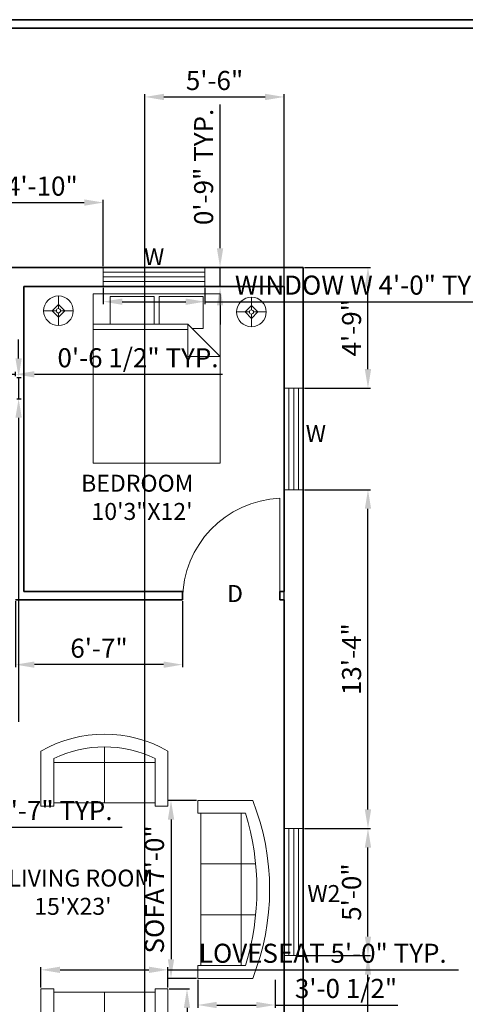
# Model space of a CAD drawing. Units: inches. Extents: x 2396 to 4051, y 1419 to 2191.
# Tile 5 of 7: x 2770 to 2981, y 1726 to 2191. Entities that reach past the tile are written whole.
import ezdxf

# ---------------------------------------------------------------- set-up
doc = ezdxf.new("R2010")
doc.units = ezdxf.units.IN
doc.layers.add('A-ANNO-TEXT', color=114, linetype='Continuous', lineweight=18, true_color=0x139b48)
doc.layers.add('A-GLAZ', color=52, linetype='Continuous', lineweight=18, true_color=0xc8c92d)
for name, color, linetype, lineweight in [('A-ANNO-TTLB', 7, 'Continuous', 35), ('A-AREA-IDEN', 6, 'Continuous', 18), ('A-DOOR', 4, 'Continuous', 18), ('A-FURN', 8, 'Continuous', 18), ('A-WALL', 7, 'Continuous', 35), ('S-ANNO-DIMS', 2, 'Continuous', 18)]:
    doc.layers.add(name, color=color, linetype=linetype, lineweight=lineweight)
doc.styles.get("Standard").update_dxf_attribs({"font": 'arial.ttf'})
doc.dimstyles.new('ISO-25', dxfattribs={"dimtxt": 9, "dimasz": 9, "dimexe": 1.25, "dimexo": 0.625, "dimgap": 2, "dimtad": 1, "dimdec": 1, "dimlunit": 4, "dimtxsty": 'Standard', "dimcen": 2.5, "dimadec": 0, "dimazin": 0, "dimtfac": 1, "dimtdec": 1, "dimtmove": 0, "dimatfit": 3, "dimfxl": 1, "dimarcsym": 0})

# ---------------------------------------------------------------- blocks, each defined once
blk = doc.blocks.new('Sofa - Roundback 7 ft.')
for p, q in [((-12.00002, -32.4421), (-12.00003, -6.5971)), ((11.99997, -32.4421), (11.99998, -6.5971)), ((-36.000027, -34), (-36.000027, -11.4696)), ((-35.999844, -13.3819), (35.9998, -13.3819)), ((35.99998, -34), (35.99998, -11.4696)), ((-36.000027, -32.4421), (35.99998, -32.4421))]:
    blk.add_line(p, q)
for points in [[(-36.000027, -34), (-42.000027, -34), (-42.000027, -8)], [(41.99998, -8), (41.99998, -34), (35.99998, -34)]]:
    blk.add_lwpolyline(points)
for centre, radius, start, end in [((0, -114.25), 114.25, 68.43141, 111.5686), ((-0.00001, -127.1968), 121.1968, 72.72033, 107.2797)]:
    blk.add_arc(centre, radius, start, end)
blk = doc.blocks.new('Sofa - Roundback Loveseat 5 ft.')
for p, q in [((0, -32.44198), (0, -5.99998)), ((-24, -33.99998), (-24, -11.46958)), ((-23.9998, -13.38178), (23.99986, -13.38178)), ((24.00004, -33.99998), (24.00004, -11.46958)), ((-24, -32.44198), (24.00004, -32.44198))]:
    blk.add_line(p, q)
for points in [[(-24, -33.99998), (-30, -33.99998), (-30, -7.99998)], [(30.00004, -7.99998), (30.00004, -33.99998), (24.00004, -33.99998)]]:
    blk.add_lwpolyline(points)
for centre, radius, start, end in [((0, -60.24998), 60.24998, 60.13715, 119.8628), ((0, -61.38438), 55.38444, 64.32083, 115.6792)]:
    blk.add_arc(centre, radius, start, end)
blk = doc.blocks.new('Bed - Queen')
for p, q in [((0, -80.00003), (0, 0)), ((0, 0), (59.99999, 0)), ((59.99999, 0), (59.99999, -80.00003)), ((7.99999, -1.2), (28.79998, -1.2)), ((7.99999, -14.4), (7.99999, -1.2)), ((28.79998, -1.2), (28.79998, -14.4)), ((31.19999, -1.2), (51.99999, -1.2)), ((31.19999, -14.4), (31.19999, -1.2)), ((51.99999, -1.2), (51.99999, -16.4)), ((0, -14.4), (44.8, -14.4)), ((44.8, -16.8), (0, -16.8)), ((59.99999, -29.6), (44.8, -14.4)), ((44.8, -14.4), (44.8, -29.6)), ((51.99999, -16.4), (46.79936, -16.4)), ((44.8, -29.6), (59.99999, -29.6)), ((59.99999, -80.00003), (0, -80.00003))]:
    blk.add_line(p, q)
blk = doc.blocks.new('Lamp - Table')
for p, q in [((0, 7), (0, 1)), ((-1, 0), (-7, 0)), ((0, 3), (-3, 0)), ((-3, 0), (0, -3)), ((3, 0), (0, 3)), ((0, -3), (3, 0)), ((1, 0), (7, 0)), ((0, -1), (0, -7))]:
    blk.add_line(p, q)
for radius in [7, 1]:
    blk.add_circle((0, 0), radius)
blk = doc.blocks.new('WIN-W-48IN')
for p, q in [((0, 0), (0, 9)), ((0, 6.75), (48, 6.75)), ((48, 0), (48, 9)), ((0, 4.5), (48, 4.5)), ((0, 2.25), (48, 2.25))]:
    blk.add_line(p, q)
blk = doc.blocks.new('DOOR-D-48IN')
blk.add_line((0, 0), (0, 48))
blk.add_arc((-2.04, 0), 48.04, 0, 87.5622)
blk = doc.blocks.new('*D42')
at = {"layer": 'Defpoints', "color": 0, "transparency": 16777216}
for p in [(2809.48, 2065.3), (2857.48, 2065.3), (2857.48, 2058.1)]:
    blk.add_point(p, dxfattribs=at)
at = {"layer": 'S-ANNO-DIMS', "color": 0, "lineweight": -2, "transparency": 16777216}
for p, q in [((2809.48, 2064.68), (2809.48, 2056.85)), ((2857.48, 2064.68), (2857.48, 2056.85)), ((2818.48, 2058.1), (2848.48, 2058.1)), ((2857.48, 2058.1), (2999.73, 2058.1))]:
    blk.add_line(p, q, dxfattribs=at)
at = {"layer": 'S-ANNO-DIMS', "color": 0, "transparency": 16777216}
for points in [[(2818.48, 2059.6), (2818.48, 2056.6), (2809.48, 2058.1)], [(2848.48, 2059.6), (2848.48, 2056.6), (2857.48, 2058.1)]]:
    blk.add_solid(points, dxfattribs=at)
at = {"layer": 'S-ANNO-DIMS', "color": 0, "transparency": 16777216, "insert": (2933.11, 2064.76), "char_height": 9, "attachment_point": 5}
blk.add_mtext('WINDOW W 4\'-0" TYP.', dxfattribs=at)
blk = doc.blocks.new('*D43')
at = {"layer": 'Defpoints', "color": 0, "transparency": 16777216}
for p in [(2857.48, 2074.3), (2864.68, 2074.3), (2857.48, 2065.3)]:
    blk.add_point(p, dxfattribs=at)
at = {"layer": 'S-ANNO-DIMS', "color": 0, "lineweight": -2, "transparency": 16777216}
for p, q in [((2864.68, 2083.3), (2864.68, 2151.16)), ((2858.11, 2074.3), (2865.93, 2074.3)), ((2864.68, 2065.3), (2864.68, 2074.3)), ((2858.11, 2065.3), (2865.93, 2065.3)), ((2864.68, 2056.3), (2864.68, 2047.3))]:
    blk.add_line(p, q, dxfattribs=at)
at = {"layer": 'S-ANNO-DIMS', "color": 0, "transparency": 16777216}
for points in [[(2863.18, 2083.3), (2866.18, 2083.3), (2864.68, 2074.3)], [(2863.18, 2056.3), (2866.18, 2056.3), (2864.68, 2065.3)]]:
    blk.add_solid(points, dxfattribs=at)
at = {"layer": 'S-ANNO-DIMS', "color": 0, "transparency": 16777216, "insert": (2858.09, 2121.73), "char_height": 9, "attachment_point": 5, "rotation": 90}
blk.add_mtext('0\'-9" TYP.', dxfattribs=at)
blk = doc.blocks.new('*D44')
at = {"layer": 'Defpoints', "color": 0, "transparency": 16777216}
for p in [(2840.06, 1742.59), (2780.06, 1733.59), (2840.06, 1733.59)]:
    blk.add_point(p, dxfattribs=at)
at = {"layer": 'S-ANNO-DIMS', "color": 0, "lineweight": -2, "transparency": 16777216}
for p, q in [((2780.06, 1734.22), (2780.06, 1743.84)), ((2840.06, 1734.22), (2840.06, 1743.84)), ((2789.06, 1742.59), (2831.06, 1742.59)), ((2840.06, 1742.59), (2977.4, 1742.59))]:
    blk.add_line(p, q, dxfattribs=at)
at = {"layer": 'S-ANNO-DIMS', "color": 0, "transparency": 16777216}
for points in [[(2789.06, 1744.09), (2789.06, 1741.09), (2780.06, 1742.59)], [(2831.06, 1744.09), (2831.06, 1741.09), (2840.06, 1742.59)]]:
    blk.add_solid(points, dxfattribs=at)
at = {"layer": 'S-ANNO-DIMS', "color": 0, "transparency": 16777216, "insert": (2913.23, 1749.25), "char_height": 9, "attachment_point": 5}
blk.add_mtext('LOVESEAT 5\'-0" TYP.', dxfattribs=at)
blk = doc.blocks.new('*D45')
at = {"layer": 'Defpoints', "color": 0, "transparency": 16777216}
for p in [(2840.06, 1733.59), (2840.06, 1696.93), (2849.06, 1696.93)]:
    blk.add_point(p, dxfattribs=at)
at = {"layer": 'S-ANNO-DIMS', "color": 0, "lineweight": -2, "transparency": 16777216}
for p, q in [((2840.69, 1733.59), (2850.31, 1733.59)), ((2849.06, 1724.59), (2849.06, 1705.93)), ((2840.69, 1696.93), (2850.31, 1696.93)), ((2849.06, 1696.93), (2849.06, 1608.1))]:
    blk.add_line(p, q, dxfattribs=at)
at = {"layer": 'S-ANNO-DIMS', "color": 0, "transparency": 16777216}
for points in [[(2847.56, 1724.59), (2850.56, 1724.59), (2849.06, 1733.59)], [(2847.56, 1705.93), (2850.56, 1705.93), (2849.06, 1696.93)]]:
    blk.add_solid(points, dxfattribs=at)
at = {"layer": 'S-ANNO-DIMS', "color": 0, "transparency": 16777216, "insert": (2842.41, 1648.02), "char_height": 9, "attachment_point": 5, "rotation": 90}
blk.add_mtext('3\'-0 1/2" TYP.', dxfattribs=at)
blk = doc.blocks.new('*D50')
at = {"layer": 'Defpoints', "color": 0, "transparency": 16777216}
for p in [(2767.98, 2022.3), (2767.98, 2012.3), (2769.48, 2012.3)]:
    blk.add_point(p, dxfattribs=at)
at = {"layer": 'S-ANNO-DIMS', "color": 0, "lineweight": -2, "transparency": 16777216}
for p, q in [((2769.48, 2031.3), (2769.48, 2040.3)), ((2768.61, 2022.3), (2770.73, 2022.3)), ((2769.48, 2022.3), (2769.48, 2012.3)), ((2768.61, 2012.3), (2770.73, 2012.3)), ((2769.48, 2003.3), (2769.48, 1859.68))]:
    blk.add_line(p, q, dxfattribs=at)
at = {"layer": 'S-ANNO-DIMS', "color": 0, "transparency": 16777216}
for points in [[(2767.98, 2031.3), (2770.98, 2031.3), (2769.48, 2022.3)], [(2767.98, 2003.3), (2770.98, 2003.3), (2769.48, 2012.3)]]:
    blk.add_solid(points, dxfattribs=at)
at = {"layer": 'S-ANNO-DIMS', "color": 0, "transparency": 16777216, "insert": (2762.83, 1926.99), "char_height": 9, "attachment_point": 5, "rotation": 90}
blk.add_mtext('BASIN TAP 0\'-10" TYP.', dxfattribs=at)
blk = doc.blocks.new('*D51')
at = {"layer": 'Defpoints', "color": 0, "transparency": 16777216}
for p in [(2767.98, 2023.8), (2761.48, 2022.3), (2767.98, 2022.3)]:
    blk.add_point(p, dxfattribs=at)
at = {"layer": 'S-ANNO-DIMS', "color": 0, "lineweight": -2, "transparency": 16777216}
for p, q in [((2752.48, 2023.8), (2743.48, 2023.8)), ((2761.48, 2022.93), (2761.48, 2025.05)), ((2761.48, 2023.8), (2767.98, 2023.8)), ((2767.98, 2022.93), (2767.98, 2025.05)), ((2776.98, 2023.8), (2865.81, 2023.8))]:
    blk.add_line(p, q, dxfattribs=at)
at = {"layer": 'S-ANNO-DIMS', "color": 0, "transparency": 16777216}
for points in [[(2752.48, 2025.3), (2752.48, 2022.3), (2761.48, 2023.8)], [(2776.98, 2025.3), (2776.98, 2022.3), (2767.98, 2023.8)]]:
    blk.add_solid(points, dxfattribs=at)
at = {"layer": 'S-ANNO-DIMS', "color": 0, "transparency": 16777216, "insert": (2825.9, 2030.45), "char_height": 9, "attachment_point": 5}
blk.add_mtext('0\'-6 1/2" TYP.', dxfattribs=at)
blk = doc.blocks.new('*D60')
at = {"layer": 'Defpoints', "color": 0, "transparency": 16777216}
for p in [(2646.98, 1816.44), (2690.18, 1816.44), (2690.18, 1809.96)]:
    blk.add_point(p, dxfattribs=at)
at = {"layer": 'S-ANNO-DIMS', "color": 0, "lineweight": -2, "transparency": 16777216}
for p, q in [((2646.98, 1815.82), (2646.98, 1808.71)), ((2690.18, 1815.82), (2690.18, 1808.71)), ((2655.98, 1809.96), (2681.18, 1809.96)), ((2690.18, 1809.96), (2818.37, 1809.96))]:
    blk.add_line(p, q, dxfattribs=at)
at = {"layer": 'S-ANNO-DIMS', "color": 0, "transparency": 16777216}
for points in [[(2655.98, 1811.46), (2655.98, 1808.46), (2646.98, 1809.96)], [(2681.18, 1811.46), (2681.18, 1808.46), (2690.18, 1809.96)]]:
    blk.add_solid(points, dxfattribs=at)
at = {"layer": 'S-ANNO-DIMS', "color": 0, "transparency": 16777216, "insert": (2758.78, 1816.62), "char_height": 9, "attachment_point": 5}
blk.add_mtext('DOOR D2 3\'-7" TYP.', dxfattribs=at)
blk = doc.blocks.new('*D62')
at = {"layer": 'Defpoints', "color": 0, "transparency": 16777216}
for p in [(2854.1, 1822.57), (2841.5, 1738.57), (2854.1, 1738.57)]:
    blk.add_point(p, dxfattribs=at)
at = {"layer": 'S-ANNO-DIMS', "color": 0, "lineweight": -2, "transparency": 16777216}
for p, q in [((2853.48, 1822.57), (2840.25, 1822.57)), ((2841.5, 1813.57), (2841.5, 1747.57)), ((2853.48, 1738.57), (2840.25, 1738.57))]:
    blk.add_line(p, q, dxfattribs=at)
at = {"layer": 'S-ANNO-DIMS', "color": 0, "transparency": 16777216}
for points in [[(2840, 1813.57), (2843, 1813.57), (2841.5, 1822.57)], [(2840, 1747.57), (2843, 1747.57), (2841.5, 1738.57)]]:
    blk.add_solid(points, dxfattribs=at)
at = {"layer": 'S-ANNO-DIMS', "color": 0, "transparency": 16777216, "insert": (2834.84, 1780.57), "char_height": 9, "attachment_point": 5, "rotation": 90}
blk.add_mtext('SOFA 7\'-0"', dxfattribs=at)
blk = doc.blocks.new('*D63')
at = {"layer": 'Defpoints', "color": 0, "transparency": 16777216}
for p in [(2854.1, 1738.57), (2890.77, 1738.57), (2890.77, 1725.97)]:
    blk.add_point(p, dxfattribs=at)
at = {"layer": 'S-ANNO-DIMS', "color": 0, "lineweight": -2, "transparency": 16777216}
for p, q in [((2854.1, 1737.94), (2854.1, 1724.72)), ((2890.77, 1737.94), (2890.77, 1724.72)), ((2863.1, 1725.97), (2881.77, 1725.97)), ((2890.77, 1725.97), (2948.66, 1725.97))]:
    blk.add_line(p, q, dxfattribs=at)
at = {"layer": 'S-ANNO-DIMS', "color": 0, "transparency": 16777216}
for points in [[(2863.1, 1727.47), (2863.1, 1724.47), (2854.1, 1725.97)], [(2881.77, 1727.47), (2881.77, 1724.47), (2890.77, 1725.97)]]:
    blk.add_solid(points, dxfattribs=at)
at = {"layer": 'S-ANNO-DIMS', "color": 0, "transparency": 16777216, "insert": (2924.21, 1732.63), "char_height": 9, "attachment_point": 5}
blk.add_mtext('3\'-0 1/2"', dxfattribs=at)
blk = doc.blocks.new('*D77')
at = {"layer": 'Defpoints', "color": 0, "transparency": 16777216}
for p in [(2529.98, 2074.3), (2499.38, 1534.3), (2774.98, 1534.3)]:
    blk.add_point(p, dxfattribs=at)
at = {"layer": 'S-ANNO-DIMS', "color": 0, "lineweight": -2, "transparency": 16777216}
for p, q in [((2529.36, 2074.3), (2498.13, 2074.3)), ((2499.38, 2065.3), (2499.38, 1543.3)), ((2774.36, 1534.3), (2498.13, 1534.3))]:
    blk.add_line(p, q, dxfattribs=at)
at = {"layer": 'S-ANNO-DIMS', "color": 0, "transparency": 16777216}
for points in [[(2497.88, 2065.3), (2500.88, 2065.3), (2499.38, 2074.3)], [(2497.88, 1543.3), (2500.88, 1543.3), (2499.38, 1534.3)]]:
    blk.add_solid(points, dxfattribs=at)
at = {"layer": 'S-ANNO-DIMS', "color": 0, "transparency": 16777216, "insert": (2492.79, 1804.3), "char_height": 9, "attachment_point": 5, "rotation": 90}
blk.add_mtext('45\'-0"', dxfattribs=at)
blk = doc.blocks.new('*D81')
at = {"layer": 'Defpoints', "color": 0, "transparency": 16777216}
for p in [(2903.98, 1809.3), (2934.58, 1809.3), (2903.98, 1749.3)]:
    blk.add_point(p, dxfattribs=at)
at = {"layer": 'S-ANNO-DIMS', "color": 0, "lineweight": -2, "transparency": 16777216}
for p, q in [((2904.61, 1809.3), (2935.83, 1809.3)), ((2934.58, 1758.3), (2934.58, 1800.3)), ((2904.61, 1749.3), (2935.83, 1749.3))]:
    blk.add_line(p, q, dxfattribs=at)
at = {"layer": 'S-ANNO-DIMS', "color": 0, "transparency": 16777216}
for points in [[(2933.08, 1800.3), (2936.08, 1800.3), (2934.58, 1809.3)], [(2933.08, 1758.3), (2936.08, 1758.3), (2934.58, 1749.3)]]:
    blk.add_solid(points, dxfattribs=at)
at = {"layer": 'S-ANNO-DIMS', "color": 0, "transparency": 16777216, "insert": (2927.99, 1779.3), "char_height": 9, "attachment_point": 5, "rotation": 90}
blk.add_mtext('5\'-0"', dxfattribs=at)
blk = doc.blocks.new('*D82')
at = {"layer": 'Defpoints', "color": 0, "transparency": 16777216}
for p in [(2903.98, 1749.3), (2934.58, 1749.3), (2903.98, 1611.9)]:
    blk.add_point(p, dxfattribs=at)
at = {"layer": 'S-ANNO-DIMS', "color": 0, "lineweight": -2, "transparency": 16777216}
for p, q in [((2904.61, 1749.3), (2935.83, 1749.3)), ((2934.58, 1620.9), (2934.58, 1740.3)), ((2904.61, 1611.9), (2935.83, 1611.9))]:
    blk.add_line(p, q, dxfattribs=at)
at = {"layer": 'S-ANNO-DIMS', "color": 0, "transparency": 16777216}
for points in [[(2933.08, 1740.3), (2936.08, 1740.3), (2934.58, 1749.3)], [(2933.08, 1620.9), (2936.08, 1620.9), (2934.58, 1611.9)]]:
    blk.add_solid(points, dxfattribs=at)
at = {"layer": 'S-ANNO-DIMS', "color": 0, "transparency": 16777216, "insert": (2927.93, 1680.6), "char_height": 9, "attachment_point": 5, "rotation": 90}
blk.add_mtext('11\'-5 1/2"', dxfattribs=at)
blk = doc.blocks.new('*D83')
at = {"layer": 'Defpoints', "color": 0, "transparency": 16777216}
for p in [(2903.98, 1969.3), (2934.58, 1969.3), (2903.98, 1809.3)]:
    blk.add_point(p, dxfattribs=at)
at = {"layer": 'S-ANNO-DIMS', "color": 0, "lineweight": -2, "transparency": 16777216}
for p, q in [((2904.61, 1969.3), (2935.83, 1969.3)), ((2934.58, 1818.3), (2934.58, 1960.3)), ((2904.61, 1809.3), (2935.83, 1809.3))]:
    blk.add_line(p, q, dxfattribs=at)
at = {"layer": 'S-ANNO-DIMS', "color": 0, "transparency": 16777216}
for points in [[(2933.08, 1960.3), (2936.08, 1960.3), (2934.58, 1969.3)], [(2933.08, 1818.3), (2936.08, 1818.3), (2934.58, 1809.3)]]:
    blk.add_solid(points, dxfattribs=at)
at = {"layer": 'S-ANNO-DIMS', "color": 0, "transparency": 16777216, "insert": (2927.99, 1889.3), "char_height": 9, "attachment_point": 5, "rotation": 90}
blk.add_mtext('13\'-4"', dxfattribs=at)
blk = doc.blocks.new('*D84')
at = {"layer": 'Defpoints', "color": 0, "transparency": 16777216}
for p in [(2903.98, 2074.3), (2934.58, 2074.3), (2903.98, 2017.3)]:
    blk.add_point(p, dxfattribs=at)
at = {"layer": 'S-ANNO-DIMS', "color": 0, "lineweight": -2, "transparency": 16777216}
for p, q in [((2904.61, 2074.3), (2935.83, 2074.3)), ((2934.58, 2026.3), (2934.58, 2065.3)), ((2904.61, 2017.3), (2935.83, 2017.3))]:
    blk.add_line(p, q, dxfattribs=at)
at = {"layer": 'S-ANNO-DIMS', "color": 0, "transparency": 16777216}
for points in [[(2933.08, 2065.3), (2936.08, 2065.3), (2934.58, 2074.3)], [(2933.08, 2026.3), (2936.08, 2026.3), (2934.58, 2017.3)]]:
    blk.add_solid(points, dxfattribs=at)
at = {"layer": 'S-ANNO-DIMS', "color": 0, "transparency": 16777216, "insert": (2927.99, 2045.8), "char_height": 9, "attachment_point": 5, "rotation": 90}
blk.add_mtext('4\'-9"', dxfattribs=at)
blk = doc.blocks.new('*D87')
at = {"layer": 'Defpoints', "color": 0, "transparency": 16777216}
for p in [(2809.48, 2104.9), (2751.48, 2074.3), (2809.48, 2074.3)]:
    blk.add_point(p, dxfattribs=at)
at = {"layer": 'S-ANNO-DIMS', "color": 0, "lineweight": -2, "transparency": 16777216}
for p, q in [((2751.48, 2074.93), (2751.48, 2106.15)), ((2760.48, 2104.9), (2800.48, 2104.9)), ((2809.48, 2074.93), (2809.48, 2106.15))]:
    blk.add_line(p, q, dxfattribs=at)
at = {"layer": 'S-ANNO-DIMS', "color": 0, "transparency": 16777216}
for points in [[(2760.48, 2106.4), (2760.48, 2103.4), (2751.48, 2104.9)], [(2800.48, 2106.4), (2800.48, 2103.4), (2809.48, 2104.9)]]:
    blk.add_solid(points, dxfattribs=at)
at = {"layer": 'S-ANNO-DIMS', "color": 0, "transparency": 16777216, "insert": (2780.48, 2111.5), "char_height": 9, "attachment_point": 5}
blk.add_mtext('4\'-10"', dxfattribs=at)
blk = doc.blocks.new('*D94')
at = {"layer": 'Defpoints', "color": 0, "transparency": 16777216}
for p in [(2767.98, 1917.3), (2846.98, 1917.3), (2767.98, 1886.7)]:
    blk.add_point(p, dxfattribs=at)
at = {"layer": 'S-ANNO-DIMS', "color": 0, "lineweight": -2, "transparency": 16777216}
for p, q in [((2767.98, 1916.68), (2767.98, 1885.45)), ((2846.98, 1916.68), (2846.98, 1885.45)), ((2837.98, 1886.7), (2776.98, 1886.7))]:
    blk.add_line(p, q, dxfattribs=at)
at = {"layer": 'S-ANNO-DIMS', "color": 0, "transparency": 16777216}
for points in [[(2776.98, 1888.2), (2776.98, 1885.2), (2767.98, 1886.7)], [(2837.98, 1888.2), (2837.98, 1885.2), (2846.98, 1886.7)]]:
    blk.add_solid(points, dxfattribs=at)
at = {"layer": 'S-ANNO-DIMS', "color": 0, "transparency": 16777216, "insert": (2807.48, 1893.3), "char_height": 9, "attachment_point": 5}
blk.add_mtext('6\'-7"', dxfattribs=at)
blk = doc.blocks.new('*D96')
at = {"layer": 'Defpoints', "color": 0, "transparency": 16777216}
for p in [(2894.98, 2154.77), (2829.18, 1641.3), (2894.98, 1641.3)]:
    blk.add_point(p, dxfattribs=at)
at = {"layer": 'S-ANNO-DIMS', "color": 0, "lineweight": -2, "transparency": 16777216}
for p, q in [((2829.18, 1641.93), (2829.18, 2156.02)), ((2838.18, 2154.77), (2885.98, 2154.77)), ((2894.98, 1641.93), (2894.98, 2156.02))]:
    blk.add_line(p, q, dxfattribs=at)
at = {"layer": 'S-ANNO-DIMS', "color": 0, "transparency": 16777216}
for points in [[(2838.18, 2156.27), (2838.18, 2153.27), (2829.18, 2154.77)], [(2885.98, 2156.27), (2885.98, 2153.27), (2894.98, 2154.77)]]:
    blk.add_solid(points, dxfattribs=at)
at = {"layer": 'S-ANNO-DIMS', "color": 0, "transparency": 16777216, "insert": (2862.08, 2161.37), "char_height": 9, "attachment_point": 5}
blk.add_mtext('5\'-6"', dxfattribs=at)

msp = doc.modelspace()

# ---------------------------------------------------------------- linework, layer by layer
at = {"layer": 'A-ANNO-TTLB'}
for points in [[(2460.66, 2191.26), (4051.21, 2191.26), (4051.21, 1469.82), (2460.66, 1469.82)], [(2464.66, 2187.26), (4047.21, 2187.26), (4047.21, 1473.82), (2464.66, 1473.82)]]:
    msp.add_lwpolyline(points, close=True, dxfattribs=at)
at = {"layer": 'A-GLAZ'}
for p, q in [((2894.98, 1809.3), (2903.98, 1809.3)), ((2897.23, 1809.3), (2897.23, 1749.3)), ((2899.48, 1809.3), (2899.48, 1749.3)), ((2901.73, 1809.3), (2901.73, 1749.3)), ((2894.98, 1749.3), (2903.98, 1749.3))]:
    msp.add_line(p, q, dxfattribs=at)
at = {"layer": 'A-WALL'}
for p, q in [((2529.98, 2074.3), (2903.98, 2074.3)), ((2903.98, 2074.3), (2903.98, 1534.3)), ((2771.98, 2065.3), (2771.98, 1921.3)), ((2771.98, 2065.3), (2894.98, 2065.3)), ((2894.98, 2065.3), (2894.98, 1921.3)), ((2846.98, 1921.3), (2771.98, 1921.3)), ((2846.98, 1917.3), (2846.98, 1921.3)), ((2894.98, 1921.3), (2892.98, 1921.3)), ((2892.98, 1917.3), (2892.98, 1921.3)), ((2846.98, 1917.3), (2767.98, 1917.3)), ((2894.98, 1917.3), (2892.98, 1917.3)), ((2894.98, 1917.3), (2894.98, 1641.3))]:
    msp.add_line(p, q, dxfattribs=at)

# ---------------------------------------------------------------- block references
at = {"layer": 'A-DOOR', "extrusion": (0, 0, -1), "zscale": -1}
msp.add_blockref('DOOR-D-48IN', (-2892.98, 1917.3), dxfattribs=at)
at = {"layer": 'A-FURN'}
for name, p in [('Lamp - Table', (2788.32, 2053.8)), ('Bed - Queen', (2804.68, 2061.81)), ('Lamp - Table', (2879.52, 2053.23)), ('Sofa - Roundback Loveseat 5 ft.', (2810.06, 1853.89))]:
    msp.add_blockref(name, p, dxfattribs=at)
at = {"layer": 'A-FURN', "rotation": 270}
msp.add_blockref('Sofa - Roundback 7 ft.', (2888.1, 1780.57), dxfattribs=at)
at = {"layer": 'A-FURN', "xscale": -1, "rotation": 180}
msp.add_blockref('Sofa - Roundback Loveseat 5 ft.', (2810.06, 1699.59), dxfattribs=at)
at = {"layer": 'A-GLAZ'}
msp.add_blockref('WIN-W-48IN', (2809.48, 2065.3), dxfattribs=at)
at = {"layer": 'A-GLAZ', "rotation": 89.99999999999781}
msp.add_blockref('WIN-W-48IN', (2903.98, 1969.3), dxfattribs=at)

# ---------------------------------------------------------------- texts
at = {"layer": 'A-ANNO-TEXT', "char_height": 8, "attachment_point": 1}
for s, insert in [('W', (2828.75, 2083.36)), ('W', (2905.16, 1999.87)), ('{D}', (2868, 1924.28)), ('W2', (2905.93, 1782.62))]:
    msp.add_mtext_dynamic_manual_height_columns(s, width=139.3028, gutter_width=12.5, heights=[0], dxfattribs=dict(at, insert=insert))
at = {"layer": 'A-AREA-IDEN', "char_height": 8, "attachment_point": 1}
for s, insert in [('      BEDROOM\\P        10\'3"X12\'', (2784.35, 1976.38)), ("   LIVING ROOM\\P        15'X23'", (2757.3, 1789.91))]:
    msp.add_mtext_dynamic_manual_height_columns(s, width=139.3028, gutter_width=12.5, heights=[0], dxfattribs=dict(at, insert=insert))

# ---------------------------------------------------------------- dimensions: what is measured, and where the dimension line sits
at = {"layer": 'S-ANNO-DIMS'}
for base, p1, p2, picture, middle in [((2894.98, 2154.77), (2829.18, 1641.3), (2894.98, 1641.3), '*D96', (2862.08, 2161.37)), ((2809.48, 2104.9), (2751.48, 2074.3), (2809.48, 2074.3), '*D87', (2780.48, 2111.5)), ((2890.77, 1725.97), (2854.1, 1738.57), (2890.77, 1738.57), '*D63', (2924.21, 1732.63))]:
    dim = msp.add_linear_dim(base=base, p1=p1, p2=p2, dimstyle='ISO-25', override={"dimdec": 1, "dimlfac": 1, "dimrnd": 0, "dimzin": 1, "dimdsep": 46, "dimlunit": 4, "dimfrac": 2}, dxfattribs=at)
    dim.commit()
    dim.dimension.update_dxf_attribs({"geometry": picture, "text_midpoint": middle})
for base, p1, p2, angle, text, picture, middle in [((2864.68, 2074.3), (2857.48, 2065.3), (2857.48, 2074.3), 90, '<> TYP.', '*D43', (2858.09, 2121.73)), ((2769.48, 2012.3), (2767.98, 2022.3), (2767.98, 2012.3), 270, 'BASIN TAP <> TYP.', '*D50', (2762.83, 1926.99)), ((2841.5, 1738.57), (2854.1, 1822.57), (2854.1, 1738.57), 270, 'SOFA <>', '*D62', (2834.84, 1780.57)), ((2849.06, 1696.93), (2840.06, 1733.59), (2840.06, 1696.93), 270, '<> TYP.', '*D45', (2842.41, 1648.02))]:
    dim = msp.add_linear_dim(base=base, p1=p1, p2=p2, angle=angle, text=text, dimstyle='ISO-25', override={"dimdec": 1, "dimlfac": 1, "dimrnd": 0, "dimzin": 1, "dimdsep": 46, "dimlunit": 4, "dimfrac": 2}, dxfattribs=at)
    dim.commit()
    dim.dimension.update_dxf_attribs({"geometry": picture, "text_midpoint": middle})
for base, p1, p2, text, picture, middle in [((2857.48, 2058.1), (2809.48, 2065.3), (2857.48, 2065.3), 'WINDOW W <> TYP.', '*D42', (2933.11, 2064.76)), ((2767.98, 2023.8), (2761.48, 2022.3), (2767.98, 2022.3), '<> TYP.', '*D51', (2825.9, 2030.45)), ((2690.18, 1809.96), (2646.98, 1816.44), (2690.18, 1816.44), 'DOOR D2 <> TYP.', '*D60', (2758.78, 1816.62)), ((2840.06, 1742.59), (2780.06, 1733.59), (2840.06, 1733.59), 'LOVESEAT <> TYP.', '*D44', (2913.23, 1749.25))]:
    dim = msp.add_linear_dim(base=base, p1=p1, p2=p2, text=text, dimstyle='ISO-25', override={"dimdec": 1, "dimlfac": 1, "dimrnd": 0, "dimzin": 1, "dimdsep": 46, "dimlunit": 4, "dimfrac": 2}, dxfattribs=at)
    dim.commit()
    dim.dimension.update_dxf_attribs({"geometry": picture, "text_midpoint": middle})
for base, p1, p2, angle, picture, middle in [((2499.38, 1534.3), (2529.98, 2074.3), (2774.98, 1534.3), 90, '*D77', (2492.79, 1804.3)), ((2934.58, 2074.3), (2903.98, 2017.3), (2903.98, 2074.3), 90, '*D84', (2927.99, 2045.8)), ((2934.58, 1969.3), (2903.98, 1809.3), (2903.98, 1969.3), 90, '*D83', (2927.99, 1889.3)), ((2767.98, 1886.7), (2846.98, 1917.3), (2767.98, 1917.3), 180, '*D94', (2807.48, 1893.3)), ((2934.58, 1809.3), (2903.98, 1749.3), (2903.98, 1809.3), 90, '*D81', (2927.99, 1779.3)), ((2934.58, 1749.3), (2903.98, 1611.9), (2903.98, 1749.3), 90, '*D82', (2927.93, 1680.6))]:
    dim = msp.add_linear_dim(base=base, p1=p1, p2=p2, angle=angle, dimstyle='ISO-25', override={"dimdec": 1, "dimlfac": 1, "dimrnd": 0, "dimzin": 1, "dimdsep": 46, "dimlunit": 4, "dimfrac": 2}, dxfattribs=at)
    dim.commit()
    dim.dimension.update_dxf_attribs({"geometry": picture, "text_midpoint": middle})

doc.saveas('drawing.dxf')
